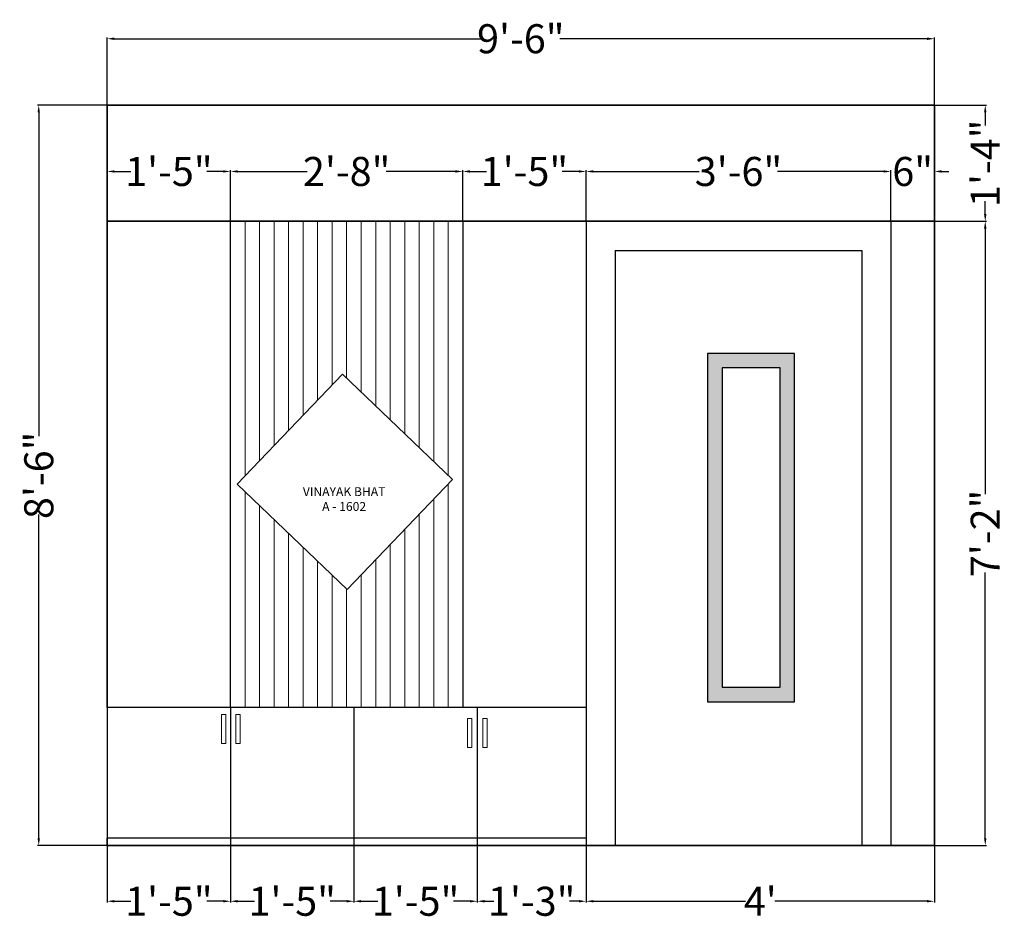
# Model space of a CAD drawing. Units: inches. Extents: x 90 to 226, y 62 to 186.
import ezdxf

# ---------------------------------------------------------------- set-up
doc = ezdxf.new("R2010")
doc.units = ezdxf.units.IN
doc.header["$MEASUREMENT"] = 0
for name, color, linetype, lineweight in [('A-ANNO-DIMS', 2, 'Continuous', 18), ('A-ANNO-TEXT', 7, 'Continuous', 18), ('A-DETL', 6, 'Continuous', 18), ('A-DOOR', 4, 'Continuous', 25), ('A-ELEV', 7, 'Continuous', 35), ('A-FURN', 8, 'Continuous', 25), ('A-FURN-GROV', 8, 'Continuous', 13), ('A-FURN-HDWR', 9, 'Continuous', 18), ('A-GLAZ-PATT', 9, 'Continuous', 13)]:
    doc.layers.add(name, color=color, linetype=linetype, lineweight=lineweight)
doc.styles.get("Standard").update_dxf_attribs({"font": 'arial.ttf'})
doc.dimstyles.get("Standard").update_dxf_attribs({"dimtxt": 4, "dimasz": 1, "dimexe": 0.18, "dimexo": 0.0625, "dimgap": 0.09, "dimtad": 0, "dimdec": 0, "dimzin": 0, "dimdsep": 46, "dimlunit": 4, "dimtxsty": 'Standard', "dimcen": 0.09, "dimadec": 0, "dimazin": 0, "dimtfac": 1, "dimtdec": 0, "dimtofl": 0, "dimtmove": 0, "dimatfit": 3, "dimfxl": 1, "dimtolj": 1, "dimtzin": 0, "dimarcsym": 0})

# ---------------------------------------------------------------- blocks, each defined once
blk = doc.blocks.new('*D1')
at = {"layer": 'A-ANNO-DIMS', "color": 0, "lineweight": -2, "transparency": 16777216}
for p, q in [((216.51, 174.2), (223.64, 174.2)), ((223.46, 173.2), (223.46, 171.42)), ((223.46, 159.2), (223.46, 160.98)), ((216.51, 158.2), (223.64, 158.2))]:
    blk.add_line(p, q, dxfattribs=at)
at = {"layer": 'A-ANNO-DIMS', "color": 0, "transparency": 16777216}
for points in [[(223.29, 173.2), (223.63, 173.2), (223.46, 174.2)], [(223.29, 159.2), (223.63, 159.2), (223.46, 158.2)]]:
    blk.add_solid(points, dxfattribs=at)
at = {"layer": 'Defpoints', "color": 0, "transparency": 16777216}
for p in [(216.45, 174.2), (216.45, 158.2), (223.46, 158.2)]:
    blk.add_point(p, dxfattribs=at)
at = {"layer": 'A-ANNO-DIMS', "color": 0, "transparency": 16777216, "insert": (223.46, 166.2), "char_height": 4, "attachment_point": 5, "rotation": 90}
blk.add_mtext('\\A1;1\'-4"', dxfattribs=at)
blk = doc.blocks.new('*D2')
at = {"layer": 'A-ANNO-DIMS', "color": 0, "lineweight": -2, "transparency": 16777216}
for p, q in [((102.45, 158.26), (102.45, 165.25)), ((103.45, 165.07), (105.73, 165.07)), ((118.45, 165.07), (116.16, 165.07)), ((119.45, 158.26), (119.45, 165.25))]:
    blk.add_line(p, q, dxfattribs=at)
at = {"layer": 'A-ANNO-DIMS', "color": 0, "transparency": 16777216}
for points in [[(103.45, 165.24), (103.45, 164.91), (102.45, 165.07)], [(118.45, 165.24), (118.45, 164.91), (119.45, 165.07)]]:
    blk.add_solid(points, dxfattribs=at)
at = {"layer": 'Defpoints', "color": 0, "transparency": 16777216}
for p in [(119.45, 165.07), (102.45, 158.2), (119.45, 158.2)]:
    blk.add_point(p, dxfattribs=at)
at = {"layer": 'A-ANNO-DIMS', "color": 0, "transparency": 16777216, "insert": (110.95, 165.07), "char_height": 4, "attachment_point": 5}
blk.add_mtext('\\A1;1\'-5"', dxfattribs=at)
blk = doc.blocks.new('*D3')
at = {"layer": 'A-ANNO-DIMS', "color": 0, "lineweight": -2, "transparency": 16777216}
for p, q in [((119.45, 158.26), (119.45, 165.25)), ((120.45, 165.07), (130, 165.07)), ((150.45, 165.07), (140.89, 165.07)), ((151.45, 158.26), (151.45, 165.25))]:
    blk.add_line(p, q, dxfattribs=at)
at = {"layer": 'A-ANNO-DIMS', "color": 0, "transparency": 16777216}
for points in [[(120.45, 165.24), (120.45, 164.91), (119.45, 165.07)], [(150.45, 165.24), (150.45, 164.91), (151.45, 165.07)]]:
    blk.add_solid(points, dxfattribs=at)
at = {"layer": 'Defpoints', "color": 0, "transparency": 16777216}
for p in [(151.45, 165.07), (119.45, 158.2), (151.45, 158.2)]:
    blk.add_point(p, dxfattribs=at)
at = {"layer": 'A-ANNO-DIMS', "color": 0, "transparency": 16777216, "insert": (135.45, 165.07), "char_height": 4, "attachment_point": 5}
blk.add_mtext('\\A1;2\'-8"', dxfattribs=at)
blk = doc.blocks.new('*D4')
at = {"layer": 'A-ANNO-DIMS', "color": 0, "lineweight": -2, "transparency": 16777216}
for p, q in [((151.45, 158.26), (151.45, 165.25)), ((152.45, 165.07), (154.73, 165.07)), ((167.45, 165.07), (165.16, 165.07)), ((168.45, 158.26), (168.45, 165.25))]:
    blk.add_line(p, q, dxfattribs=at)
at = {"layer": 'A-ANNO-DIMS', "color": 0, "transparency": 16777216}
for points in [[(152.45, 165.24), (152.45, 164.91), (151.45, 165.07)], [(167.45, 165.24), (167.45, 164.91), (168.45, 165.07)]]:
    blk.add_solid(points, dxfattribs=at)
at = {"layer": 'Defpoints', "color": 0, "transparency": 16777216}
for p in [(168.45, 165.07), (151.45, 158.2), (168.45, 158.2)]:
    blk.add_point(p, dxfattribs=at)
at = {"layer": 'A-ANNO-DIMS', "color": 0, "transparency": 16777216, "insert": (159.95, 165.07), "char_height": 4, "attachment_point": 5}
blk.add_mtext('\\A1;1\'-5"', dxfattribs=at)
blk = doc.blocks.new('*D5')
at = {"layer": 'A-ANNO-DIMS', "color": 0, "lineweight": -2, "transparency": 16777216}
for p, q in [((168.45, 158.26), (168.45, 165.25)), ((169.45, 165.07), (184.04, 165.07)), ((209.45, 165.07), (194.85, 165.07)), ((210.45, 158.26), (210.45, 165.25))]:
    blk.add_line(p, q, dxfattribs=at)
at = {"layer": 'A-ANNO-DIMS', "color": 0, "transparency": 16777216}
for points in [[(169.45, 165.24), (169.45, 164.91), (168.45, 165.07)], [(209.45, 165.24), (209.45, 164.91), (210.45, 165.07)]]:
    blk.add_solid(points, dxfattribs=at)
at = {"layer": 'Defpoints', "color": 0, "transparency": 16777216}
for p in [(210.45, 165.07), (168.45, 158.2), (210.45, 158.2)]:
    blk.add_point(p, dxfattribs=at)
at = {"layer": 'A-ANNO-DIMS', "color": 0, "transparency": 16777216, "insert": (189.45, 165.07), "char_height": 4, "attachment_point": 5}
blk.add_mtext('\\A1;3\'-6"', dxfattribs=at)
blk = doc.blocks.new('*D6')
at = {"layer": 'A-ANNO-DIMS', "color": 0, "lineweight": -2, "transparency": 16777216}
for p, q in [((209.45, 165.07), (208.45, 165.07)), ((210.45, 158.26), (210.45, 165.25)), ((216.45, 158.26), (216.45, 165.25)), ((217.45, 165.07), (218.45, 165.07))]:
    blk.add_line(p, q, dxfattribs=at)
at = {"layer": 'A-ANNO-DIMS', "color": 0, "transparency": 16777216}
for points in [[(209.45, 165.24), (209.45, 164.91), (210.45, 165.07)], [(217.45, 165.24), (217.45, 164.91), (216.45, 165.07)]]:
    blk.add_solid(points, dxfattribs=at)
at = {"layer": 'Defpoints', "color": 0, "transparency": 16777216}
for p in [(216.45, 165.07), (210.45, 158.2), (216.45, 158.2)]:
    blk.add_point(p, dxfattribs=at)
at = {"layer": 'A-ANNO-DIMS', "color": 0, "transparency": 16777216, "insert": (213.45, 165.07), "char_height": 4, "attachment_point": 5}
blk.add_mtext('\\A1;6"', dxfattribs=at)
blk = doc.blocks.new('*D7')
at = {"layer": 'A-ANNO-DIMS', "color": 0, "lineweight": -2, "transparency": 16777216}
for p, q in [((102.45, 174.26), (102.45, 183.54)), ((103.45, 183.36), (154.04, 183.36)), ((215.45, 183.36), (164.85, 183.36)), ((216.45, 174.26), (216.45, 183.54))]:
    blk.add_line(p, q, dxfattribs=at)
at = {"layer": 'A-ANNO-DIMS', "color": 0, "transparency": 16777216}
for points in [[(103.45, 183.53), (103.45, 183.19), (102.45, 183.36)], [(215.45, 183.53), (215.45, 183.19), (216.45, 183.36)]]:
    blk.add_solid(points, dxfattribs=at)
at = {"layer": 'Defpoints', "color": 0, "transparency": 16777216}
for p in [(216.45, 183.36), (102.45, 174.2), (216.45, 174.2)]:
    blk.add_point(p, dxfattribs=at)
at = {"layer": 'A-ANNO-DIMS', "color": 0, "transparency": 16777216, "insert": (159.45, 183.36), "char_height": 4, "attachment_point": 5}
blk.add_mtext('\\A1;9\'-6"', dxfattribs=at)
blk = doc.blocks.new('*D8')
at = {"layer": 'A-ANNO-DIMS', "color": 0, "lineweight": -2, "transparency": 16777216}
for p, q in [((102.38, 174.2), (92.84, 174.2)), ((93.02, 173.2), (93.02, 128.61)), ((93.02, 73.2), (93.02, 117.79)), ((102.38, 72.2), (92.84, 72.2))]:
    blk.add_line(p, q, dxfattribs=at)
at = {"layer": 'A-ANNO-DIMS', "color": 0, "transparency": 16777216}
for points in [[(92.85, 173.2), (93.18, 173.2), (93.02, 174.2)], [(92.85, 73.2), (93.18, 73.2), (93.02, 72.2)]]:
    blk.add_solid(points, dxfattribs=at)
at = {"layer": 'Defpoints', "color": 0, "transparency": 16777216}
for p in [(93.02, 174.2), (102.45, 174.2), (102.45, 72.2)]:
    blk.add_point(p, dxfattribs=at)
at = {"layer": 'A-ANNO-DIMS', "color": 0, "transparency": 16777216, "insert": (93.02, 123.2), "char_height": 4, "attachment_point": 5, "rotation": 90}
blk.add_mtext('\\A1;8\'-6"', dxfattribs=at)
blk = doc.blocks.new('*D9')
at = {"layer": 'A-ANNO-DIMS', "color": 0, "lineweight": -2, "transparency": 16777216}
for p, q in [((216.51, 158.2), (223.64, 158.2)), ((223.46, 157.2), (223.46, 120.59)), ((223.46, 73.2), (223.46, 109.81)), ((216.51, 72.2), (223.64, 72.2))]:
    blk.add_line(p, q, dxfattribs=at)
at = {"layer": 'A-ANNO-DIMS', "color": 0, "transparency": 16777216}
for points in [[(223.29, 157.2), (223.63, 157.2), (223.46, 158.2)], [(223.29, 73.2), (223.63, 73.2), (223.46, 72.2)]]:
    blk.add_solid(points, dxfattribs=at)
at = {"layer": 'Defpoints', "color": 0, "transparency": 16777216}
for p in [(216.45, 158.2), (216.45, 72.2), (223.46, 72.2)]:
    blk.add_point(p, dxfattribs=at)
at = {"layer": 'A-ANNO-DIMS', "color": 0, "transparency": 16777216, "insert": (223.46, 115.2), "char_height": 4, "attachment_point": 5, "rotation": 90}
blk.add_mtext('\\A1;7\'-2"', dxfattribs=at)
blk = doc.blocks.new('*D10')
at = {"layer": 'A-ANNO-DIMS', "color": 0, "lineweight": -2, "transparency": 16777216}
for p, q in [((102.45, 73.13), (102.45, 64.33)), ((119.45, 73.13), (119.45, 64.33)), ((103.45, 64.51), (105.73, 64.51)), ((118.45, 64.51), (116.16, 64.51))]:
    blk.add_line(p, q, dxfattribs=at)
at = {"layer": 'A-ANNO-DIMS', "color": 0, "transparency": 16777216}
for points in [[(103.45, 64.68), (103.45, 64.35), (102.45, 64.51)], [(118.45, 64.68), (118.45, 64.35), (119.45, 64.51)]]:
    blk.add_solid(points, dxfattribs=at)
at = {"layer": 'Defpoints', "color": 0, "transparency": 16777216}
for p in [(102.45, 73.2), (119.45, 73.2), (119.45, 64.51)]:
    blk.add_point(p, dxfattribs=at)
at = {"layer": 'A-ANNO-DIMS', "color": 0, "transparency": 16777216, "insert": (110.95, 64.51), "char_height": 4, "attachment_point": 5}
blk.add_mtext('\\A1;1\'-5"', dxfattribs=at)
blk = doc.blocks.new('*D11')
at = {"layer": 'A-ANNO-DIMS', "color": 0, "lineweight": -2, "transparency": 16777216}
for p, q in [((119.45, 73.13), (119.45, 64.33)), ((136.45, 73.13), (136.45, 64.33)), ((120.45, 64.51), (122.73, 64.51)), ((135.45, 64.51), (133.16, 64.51))]:
    blk.add_line(p, q, dxfattribs=at)
at = {"layer": 'A-ANNO-DIMS', "color": 0, "transparency": 16777216}
for points in [[(120.45, 64.68), (120.45, 64.35), (119.45, 64.51)], [(135.45, 64.68), (135.45, 64.35), (136.45, 64.51)]]:
    blk.add_solid(points, dxfattribs=at)
at = {"layer": 'Defpoints', "color": 0, "transparency": 16777216}
for p in [(119.45, 73.2), (136.45, 73.2), (136.45, 64.51)]:
    blk.add_point(p, dxfattribs=at)
at = {"layer": 'A-ANNO-DIMS', "color": 0, "transparency": 16777216, "insert": (127.95, 64.51), "char_height": 4, "attachment_point": 5}
blk.add_mtext('\\A1;1\'-5"', dxfattribs=at)
blk = doc.blocks.new('*D12')
at = {"layer": 'A-ANNO-DIMS', "color": 0, "lineweight": -2, "transparency": 16777216}
for p, q in [((136.45, 73.13), (136.45, 64.33)), ((153.45, 73.13), (153.45, 64.33)), ((137.45, 64.51), (139.73, 64.51)), ((152.45, 64.51), (150.16, 64.51))]:
    blk.add_line(p, q, dxfattribs=at)
at = {"layer": 'A-ANNO-DIMS', "color": 0, "transparency": 16777216}
for points in [[(137.45, 64.68), (137.45, 64.35), (136.45, 64.51)], [(152.45, 64.68), (152.45, 64.35), (153.45, 64.51)]]:
    blk.add_solid(points, dxfattribs=at)
at = {"layer": 'Defpoints', "color": 0, "transparency": 16777216}
for p in [(136.45, 73.2), (153.45, 73.2), (153.45, 64.51)]:
    blk.add_point(p, dxfattribs=at)
at = {"layer": 'A-ANNO-DIMS', "color": 0, "transparency": 16777216, "insert": (144.95, 64.51), "char_height": 4, "attachment_point": 5}
blk.add_mtext('\\A1;1\'-5"', dxfattribs=at)
blk = doc.blocks.new('*D13')
at = {"layer": 'A-ANNO-DIMS', "color": 0, "lineweight": -2, "transparency": 16777216}
for p, q in [((153.45, 73.13), (153.45, 64.33)), ((168.45, 73.13), (168.45, 64.33)), ((154.45, 64.51), (155.73, 64.51)), ((167.45, 64.51), (166.16, 64.51))]:
    blk.add_line(p, q, dxfattribs=at)
at = {"layer": 'A-ANNO-DIMS', "color": 0, "transparency": 16777216}
for points in [[(154.45, 64.68), (154.45, 64.35), (153.45, 64.51)], [(167.45, 64.68), (167.45, 64.35), (168.45, 64.51)]]:
    blk.add_solid(points, dxfattribs=at)
at = {"layer": 'Defpoints', "color": 0, "transparency": 16777216}
for p in [(153.45, 73.2), (168.45, 73.2), (168.45, 64.51)]:
    blk.add_point(p, dxfattribs=at)
at = {"layer": 'A-ANNO-DIMS', "color": 0, "transparency": 16777216, "insert": (160.95, 64.51), "char_height": 4, "attachment_point": 5}
blk.add_mtext('\\A1;1\'-3"', dxfattribs=at)
blk = doc.blocks.new('*D14')
at = {"layer": 'A-ANNO-DIMS', "color": 0, "lineweight": -2, "transparency": 16777216}
for p, q in [((168.45, 72.13), (168.45, 64.33)), ((216.45, 72.13), (216.45, 64.33)), ((169.45, 64.51), (190.43, 64.51)), ((215.45, 64.51), (194.46, 64.51))]:
    blk.add_line(p, q, dxfattribs=at)
at = {"layer": 'A-ANNO-DIMS', "color": 0, "transparency": 16777216}
for points in [[(169.45, 64.68), (169.45, 64.35), (168.45, 64.51)], [(215.45, 64.68), (215.45, 64.35), (216.45, 64.51)]]:
    blk.add_solid(points, dxfattribs=at)
at = {"layer": 'Defpoints', "color": 0, "transparency": 16777216}
for p in [(168.45, 72.2), (216.45, 72.2), (216.45, 64.51)]:
    blk.add_point(p, dxfattribs=at)
at = {"layer": 'A-ANNO-DIMS', "color": 0, "transparency": 16777216, "insert": (192.45, 64.51), "char_height": 4, "attachment_point": 5}
blk.add_mtext("\\A1;4'", dxfattribs=at)
blk = doc.blocks.new('HANDLE-4IN')
blk.add_lwpolyline([(0, 0), (0.6, 0), (0.6, 4), (0, 4)], close=True)

msp = doc.modelspace()

# ---------------------------------------------------------------- hatches: boundary and pattern name
at = {"layer": 'A-GLAZ-PATT'}
h = msp.add_hatch(color=256, dxfattribs=at)
h.dxf.hatch_style = 1
h.paths.add_polyline_path([(197.19, 140.01), (185.19, 140.01), (185.19, 92.01), (197.19, 92.01)])
h.paths.add_polyline_path([(195.19, 138.01), (195.19, 94.01), (187.19, 94.01), (187.19, 138.01)], flags=16)

# ---------------------------------------------------------------- linework, layer by layer
at = {"layer": 'A-DETL'}
msp.add_lwpolyline([(150.04, 122.63), (134.87, 137.15), (120.35, 121.98), (135.52, 107.46)], close=True, dxfattribs=at)
at = {"layer": 'A-DOOR'}
for p, q in [((168.45, 158.2), (168.45, 72.2)), ((210.45, 158.2), (210.45, 72.2)), ((172.45, 154.2), (172.45, 72.2)), ((172.45, 154.2), (206.45, 154.2)), ((206.45, 154.2), (206.45, 72.2))]:
    msp.add_line(p, q, dxfattribs=at)
for points in [[(185.19, 92.01), (197.19, 92.01), (197.19, 140.01), (185.19, 140.01)], [(187.19, 94.01), (195.19, 94.01), (195.19, 138.01), (187.19, 138.01)]]:
    msp.add_lwpolyline(points, close=True, dxfattribs=at)
at = {"layer": 'A-ELEV'}
for p, q in [((102.45, 174.2), (216.45, 174.2)), ((102.45, 91.2), (102.45, 174.2)), ((216.45, 174.2), (216.45, 72.2)), ((102.45, 158.2), (216.45, 158.2)), ((102.45, 72.2), (102.45, 73.2)), ((216.45, 72.2), (102.45, 72.2))]:
    msp.add_line(p, q, dxfattribs=at)
at = {"layer": 'A-FURN'}
for p, q in [((119.45, 91.2), (119.45, 158.2)), ((151.45, 158.2), (151.45, 91.2)), ((168.45, 91.2), (102.45, 91.2)), ((102.45, 91.2), (102.45, 73.2)), ((119.45, 91.2), (119.45, 73.2)), ((136.45, 91.2), (136.45, 73.2)), ((153.45, 91.2), (153.45, 73.2)), ((168.45, 73.2), (102.45, 73.2))]:
    msp.add_line(p, q, dxfattribs=at)
at = {"layer": 'A-FURN-GROV'}
for p, q in [((121.45, 123.13), (121.45, 158.2)), ((123.45, 125.21), (123.45, 158.2)), ((125.45, 127.3), (125.45, 158.2)), ((127.45, 129.39), (127.45, 158.2)), ((129.45, 131.48), (129.45, 158.2)), ((131.45, 133.57), (131.45, 158.2)), ((133.45, 135.66), (133.45, 158.2)), ((135.45, 136.61), (135.45, 158.2)), ((137.45, 134.69), (137.45, 158.2)), ((139.45, 132.78), (139.45, 158.2)), ((141.45, 130.87), (141.45, 158.2)), ((143.45, 128.95), (143.45, 158.2)), ((145.45, 127.04), (145.45, 158.2)), ((147.45, 125.12), (147.45, 158.2)), ((149.45, 123.21), (149.45, 158.2)), ((121.45, 91.2), (121.45, 120.94)), ((149.45, 91.2), (149.45, 122.01)), ((147.45, 91.2), (147.45, 119.92)), ((123.45, 91.2), (123.45, 119.02)), ((125.45, 91.2), (125.45, 117.11)), ((145.45, 91.2), (145.45, 117.83)), ((143.45, 91.2), (143.45, 115.74)), ((127.45, 91.2), (127.45, 115.2)), ((129.45, 91.2), (129.45, 113.28)), ((141.45, 91.2), (141.45, 113.65)), ((131.45, 91.2), (131.45, 111.37)), ((139.45, 91.2), (139.45, 111.56)), ((133.45, 91.2), (133.45, 109.45)), ((137.45, 91.2), (137.45, 109.47)), ((135.45, 91.2), (135.45, 107.54))]:
    msp.add_line(p, q, dxfattribs=at)

# ---------------------------------------------------------------- block references
at = {"layer": 'A-FURN-HDWR'}
for p in [(118.18, 86.25), (120.16, 86.25), (152.1, 85.71), (154.21, 85.71)]:
    msp.add_blockref('HANDLE-4IN', p, dxfattribs=at)

# ---------------------------------------------------------------- texts
at = {"layer": 'A-ANNO-TEXT', "insert": (127.36, 121.57), "char_height": 1.227, "attachment_point": 1}
msp.add_mtext_dynamic_manual_height_columns('\\pxqc;VINAYAK BHAT\\PA - 1602', width=15.4905, gutter_width=6.13, heights=[0], dxfattribs=at)

# ---------------------------------------------------------------- dimensions: what is measured, and where the dimension line sits
at = {"layer": 'A-ANNO-DIMS'}
for base, p1, p2, picture, middle in [((216.45, 183.36), (102.45, 174.2), (216.45, 174.2), '*D7', (159.45, 183.36)), ((119.45, 165.07), (102.45, 158.2), (119.45, 158.2), '*D2', (110.95, 165.07)), ((151.45, 165.07), (119.45, 158.2), (151.45, 158.2), '*D3', (135.45, 165.07)), ((168.45, 165.07), (151.45, 158.2), (168.45, 158.2), '*D4', (159.95, 165.07)), ((210.45, 165.07), (168.45, 158.2), (210.45, 158.2), '*D5', (189.45, 165.07)), ((216.45, 165.07), (210.45, 158.2), (216.45, 158.2), '*D6', (213.45, 165.07)), ((119.45, 64.51), (102.45, 73.2), (119.45, 73.2), '*D10', (110.95, 64.51)), ((136.45, 64.51), (119.45, 73.2), (136.45, 73.2), '*D11', (127.95, 64.51)), ((153.45, 64.51), (136.45, 73.2), (153.45, 73.2), '*D12', (144.95, 64.51)), ((168.45, 64.51), (153.45, 73.2), (168.45, 73.2), '*D13', (160.95, 64.51)), ((216.45, 64.51), (168.45, 72.2), (216.45, 72.2), '*D14', (192.45, 64.51))]:
    dim = msp.add_linear_dim(base=base, p1=p1, p2=p2, dimstyle='Standard', override={"dimclrd": 0, "dimclre": 0, "dimclrt": 0}, dxfattribs=at)
    dim.commit()
    dim.dimension.update_dxf_attribs({"geometry": picture, "text_midpoint": middle})
for base, p1, p2, picture, middle in [((93.02, 174.2), (102.45, 72.2), (102.45, 174.2), '*D8', (93.02, 123.2)), ((223.46, 158.2), (216.45, 174.2), (216.45, 158.2), '*D1', (223.46, 166.2)), ((223.46, 72.2), (216.45, 158.2), (216.45, 72.2), '*D9', (223.46, 115.2))]:
    dim = msp.add_linear_dim(base=base, p1=p1, p2=p2, angle=90, dimstyle='Standard', override={"dimclrd": 0, "dimclre": 0, "dimclrt": 0}, dxfattribs=at)
    dim.commit()
    dim.dimension.update_dxf_attribs({"geometry": picture, "text_midpoint": middle})

doc.saveas('drawing.dxf')
